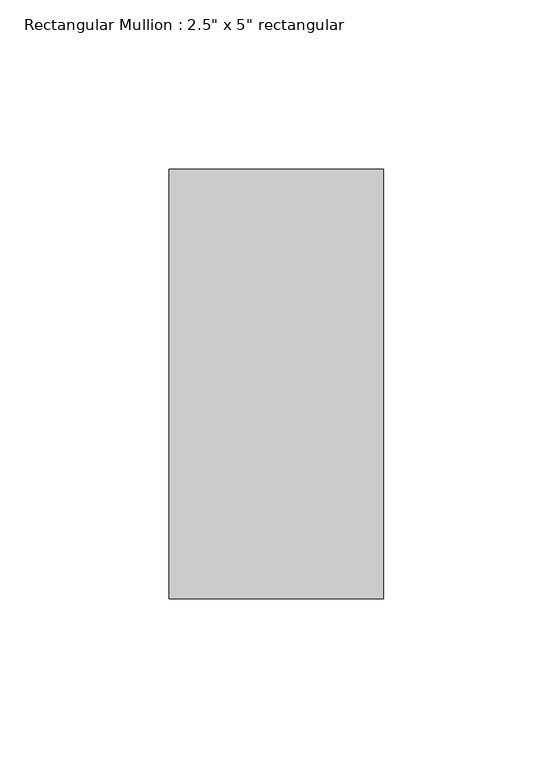
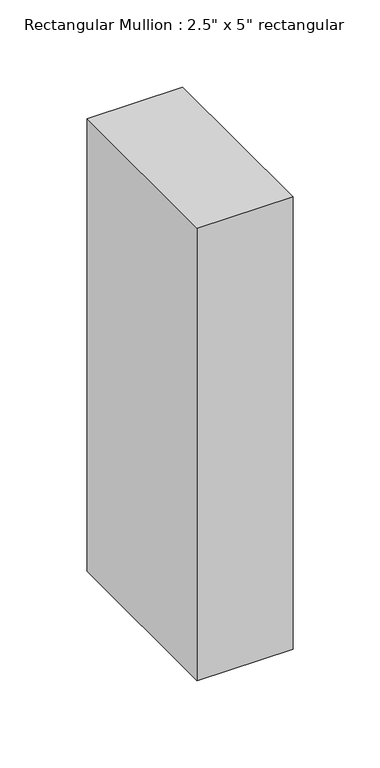
"""IFC4 building model written with IfcOpenShell, lengths in millimetres: member geometry."""

from ifc_helpers import new_model, si_unit, frame, origin, place, context, project, spatial, polyline, outline, extrude, source, transform, mapped, element, save


def member_3060f3e2(model_context):
    return source(origin(), model_context, "Body", "SweptSolid", [
        extrude(outline(polyline([(0.0, 63.5), (0.0, -63.5), (-63.5, -63.5), (-63.5, 63.5), (0.0, 63.5)])), frame((0.0, 0.0, -317.5), z_axis=(0.0, 0.0, 1.0), x_axis=(1.0, 0.0, 0.0)), (0.0, 0.0, 1.0), 317.5),
    ])


if __name__ == "__main__":
    model = new_model("IFC4")
    model_context = context("Model", 3, world=origin())
    ifc_project = project(units=[si_unit("LENGTHUNIT", "METRE", prefix="MILLI")], contexts=[model_context])
    site = spatial("IfcSite", under=ifc_project)
    building = spatial("IfcBuilding", under=site)
    placement = place(None, origin())
    member_shape = member_3060f3e2(model_context)
    element("IfcMember", 1, ObjectType="Rectangular Mullion : 2.5\" x 5\" rectangular", at=placement, inside=building, context=model_context, shape_type="MappedRepresentation", body=[
        mapped(member_shape, transform((0.0, 0.0, 0.0), x_axis=(1.0, 0.0, 0.0), y_axis=(0.0, 1.0, 0.0), z_axis=(0.0, 0.0, 1.0))),
    ])
    save(model, "model.ifc")

# Revit data of these elements
# Type "Rectangular Mullion : 2.5\" x 5\" rectangular"
#   built-in parameter 1007304 = 0.416667 (stored number, unit not read)
#   built-in parameter 1007301 = 0.104167 (stored number, unit not read)
#   built-in parameter 1007300 = 0.104167 (stored number, unit not read)
